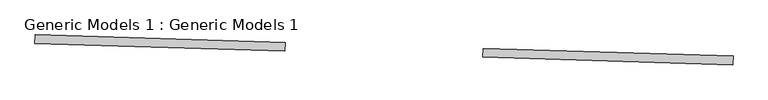
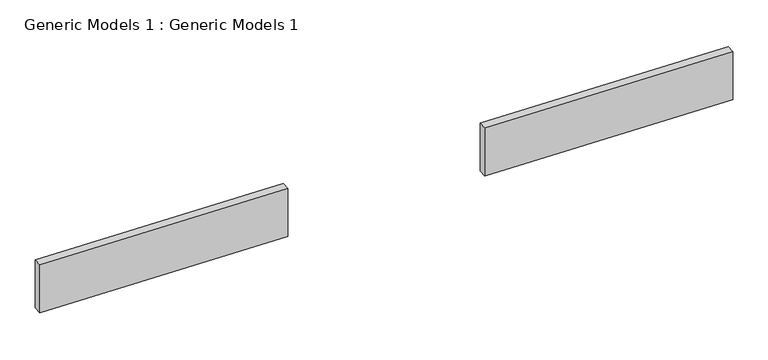
"""IFC4 building model written with IfcOpenShell, lengths in millimetres: proxy geometry, Generic Models 1 : Generic Models 1."""

from ifc_helpers import new_model, si_unit, frame, origin, place, context, project, spatial, polyline, outline, extrude, source, transform, mapped, element, save


def generic_models_1_generic_models_1_88037803(model_context):
    return source(origin(), model_context, "Body", "SweptSolid", [
        extrude(outline(polyline([(4984.7000925, -10019.4858729), (567.2123572, -9882.8613196), (571.9235487, -9730.5341563), (4989.411284, -9867.1587096), (4984.7000925, -10019.4858729)])), frame((0.0, 0.0, 316.5995699), z_axis=(0.0, 0.0, 1.0), x_axis=(1.0, 0.0, 0.0)), (0.0, 0.0, 1.0), 914.4),
        extrude(outline(polyline([(-2936.3123984, -9774.5039152), (-7353.8001337, -9637.8793618), (-7349.0889422, -9485.5521985), (-2931.6012069, -9622.1767519), (-2936.3123984, -9774.5039152)])), frame((0.0, 0.0, 316.5995699), z_axis=(0.0, 0.0, 1.0), x_axis=(1.0, 0.0, 0.0)), (0.0, 0.0, 1.0), 914.4),
    ])


if __name__ == "__main__":
    model = new_model("IFC4")
    model_context = context("Model", 3, world=origin())
    ifc_project = project(units=[si_unit("LENGTHUNIT", "METRE", prefix="MILLI")], contexts=[model_context])
    site = spatial("IfcSite", under=ifc_project)
    building = spatial("IfcBuilding", under=site)
    placement = place(None, origin())
    generic_models_1_generic_models_1_shape = generic_models_1_generic_models_1_88037803(model_context)
    element("IfcBuildingElementProxy", 1, Name="Generic Models 1 : Generic Models 1", ObjectType="Generic Models 1 : Generic Models 1", at=placement, inside=building, context=model_context, shape_type="MappedRepresentation", body=[
        mapped(generic_models_1_generic_models_1_shape, transform((0.0, 0.0, 0.0), x_axis=(1.0, 0.0, 0.0), y_axis=(0.0, 1.0, 0.0), z_axis=(0.0, 0.0, 1.0))),
    ])
    save(model, "model.ifc")

# Revit data of these elements
# Element 1 (IfcBuildingElementProxy, "Generic Models 1 : Generic Models 1")
#   Materials on its faces: "Default Mass Exterior Wall"
# Materials
#   "Default Mass Exterior Wall": class "Generic", colour RGB 133 178 44, transparency 0.2, Cost = 0
